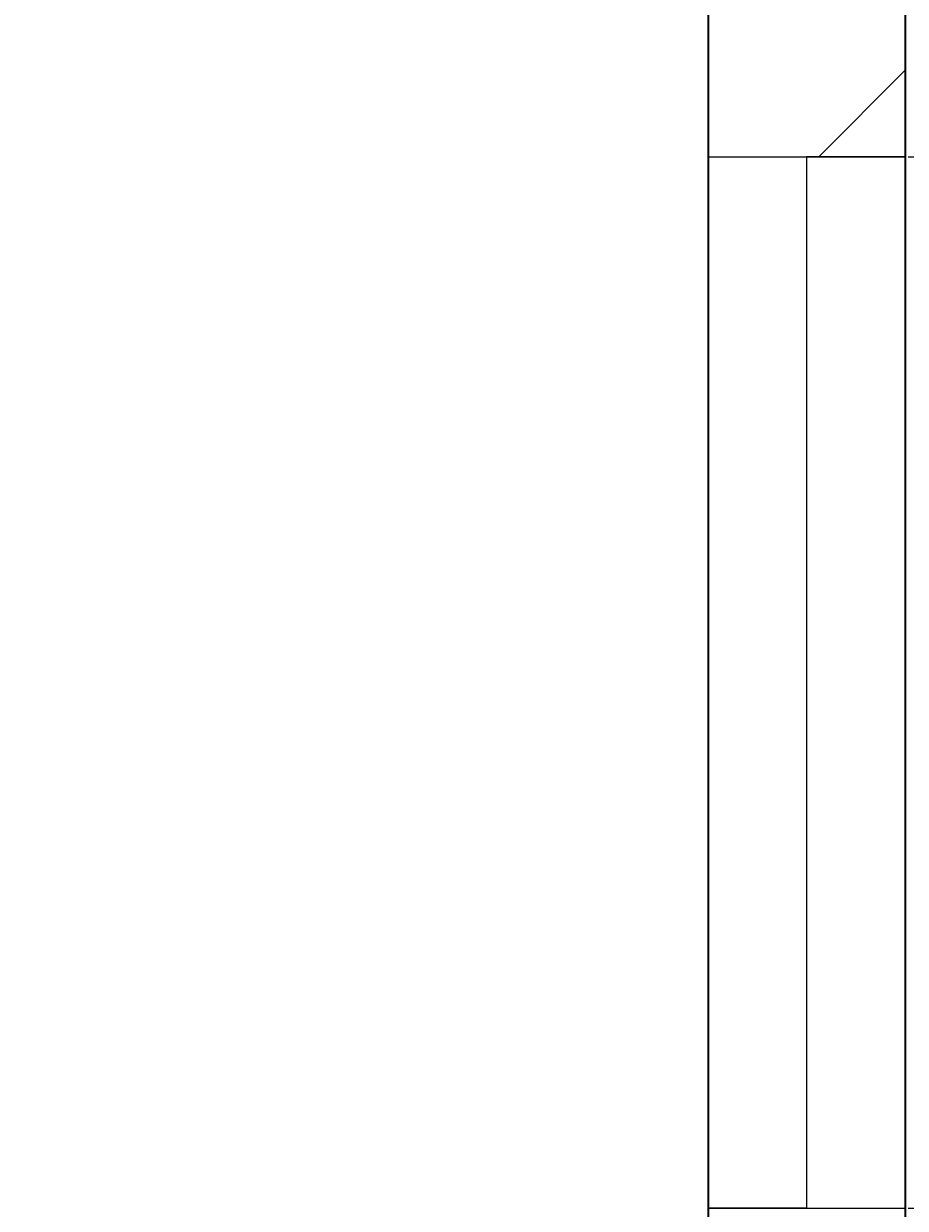
# Model space of a CAD drawing. Units: inches. Extents: x 1962 to 2771, y 1245 to 2660.
# Tile 18 of 114: x 2641 to 2661, y 1665 to 1692. Entities that reach past the tile are written whole.
import ezdxf

# ---------------------------------------------------------------- set-up
doc = ezdxf.new("R2010")
doc.units = ezdxf.units.IN
for name, color, linetype, lineweight in [('A-ANNO-DIMS', 2, 'Continuous', 18), ('A-GLAZ', 4, 'Continuous', 18), ('A-WALL', 7, 'Continuous', 35), ('A-WALL-PATT', 252, 'Continuous', 13)]:
    doc.layers.add(name, color=color, linetype=linetype, lineweight=lineweight)
doc.styles.get("Standard").update_dxf_attribs({"font": 'arial.ttf'})
doc.dimstyles.get("Standard").update_dxf_attribs({"dimtxt": 0.18, "dimasz": 0.18, "dimexe": 0.18, "dimexo": 0.0625, "dimgap": 0.09, "dimtad": 0, "dimtih": 1, "dimtoh": 1, "dimdec": 4, "dimzin": 0, "dimdsep": 46, "dimtxsty": 'Standard', "dimcen": 0.09, "dimadec": 0, "dimazin": 0, "dimtfac": 1, "dimtdec": 4, "dimtofl": 0, "dimtmove": 0, "dimatfit": 3, "dimfxl": 1, "dimtolj": 1, "dimtzin": 0, "dimarcsym": 0})

# ---------------------------------------------------------------- blocks, each defined once
blk = doc.blocks.new('WIN-24IN-A')
for p, q in [((0, 24), (4.5, 24)), ((4.5, 24), (2.25, 24)), ((2.25, 24), (2.25, 0)), ((2.25, 0), (0, 0)), ((0, 0), (4.5, 0))]:
    blk.add_line(p, q)
blk = doc.blocks.new('*D18')
at = {"layer": 'A-ANNO-DIMS', "color": 0, "lineweight": -2, "transparency": 16777216}
for p, q in [((2660.87, 1688.966), (2664.587, 1688.966)), ((2664.407, 1688.786), (2664.407, 1677.147)), ((2664.407, 1665.146), (2664.407, 1676.786)), ((2660.87, 1664.966), (2664.587, 1664.966))]:
    blk.add_line(p, q, dxfattribs=at)
at = {"layer": 'A-ANNO-DIMS', "color": 0, "transparency": 16777216}
for points in [[(2664.377, 1688.786), (2664.437, 1688.786), (2664.407, 1688.966)], [(2664.377, 1665.146), (2664.437, 1665.146), (2664.407, 1664.966)]]:
    blk.add_solid(points, dxfattribs=at)
at = {"layer": 'Defpoints', "color": 0, "transparency": 16777216}
for p in [(2660.807, 1688.966), (2664.407, 1688.966), (2660.807, 1664.966)]:
    blk.add_point(p, dxfattribs=at)
at = {"layer": 'A-ANNO-DIMS', "color": 0, "transparency": 16777216, "insert": (2664.407, 1676.966), "char_height": 0.18, "attachment_point": 5}
blk.add_mtext('\\A1;W1A 24 TYP.', dxfattribs=at)

msp = doc.modelspace()

# ---------------------------------------------------------------- hatches: boundary and pattern name
at = {"layer": 'A-WALL-PATT'}
h = msp.add_hatch(dxfattribs=at)
h.set_pattern_fill('ANSI32', color=256)
h.paths.add_polyline_path([(2090.8074, 2467.3437), (2141.6481, 2467.3437), (2141.6481, 2469.5937), (2141.6481, 2471.8437), (2086.3074, 2471.8437), (2086.3074, 2422.5333), (2090.8074, 2422.5333)])
h.paths.add_polyline_path([(2282.7664, 2471.8437), (2204.8982, 2471.8437), (2204.8982, 2467.3437), (2234.8074, 2467.3437), (2234.8074, 2311.3437), (2228.7492, 2311.3437), (2228.7492, 2306.8437), (2234.8074, 2306.8437), (2331.9227, 2306.8437), (2331.9227, 2309.0937), (2331.9227, 2311.3437), (2239.3074, 2311.3437), (2239.3074, 2467.3437), (2282.7664, 2467.3437), (2282.7664, 2469.5937)])
h.paths.add_polyline_path([(2471.4531, 2519.8437), (2552.011, 2519.8437), (2564.3996, 2519.8437), (2564.3996, 2511.1389), (2568.8996, 2511.1389), (2568.8996, 2524.3437), (2466.9531, 2524.3437), (2466.9531, 2471.8437), (2450.0749, 2471.8437), (2446.4672, 2471.8437), (2446.4672, 2467.3437), (2450.0749, 2467.3437), (2475.9988, 2467.3437), (2475.9988, 2469.5937), (2475.9988, 2471.8437), (2471.4531, 2471.8437)])
h.paths.add_polyline_path([(2575.2231, 2469.5937), (2575.2231, 2471.8437), (2568.8996, 2471.8437), (2568.8996, 2487.1389), (2564.3996, 2487.1389), (2564.3996, 2471.8437), (2556.511, 2471.8437), (2499.2904, 2471.8437), (2499.2904, 2467.3437), (2507.8074, 2467.3437), (2507.8074, 2311.3437), (2414.863, 2311.3437), (2414.863, 2306.8437), (2512.3074, 2306.8437), (2517.0114, 2306.8437), (2517.0114, 2309.0937), (2517.0114, 2311.3437), (2512.3074, 2311.3437), (2512.3074, 2467.3437), (2575.2231, 2467.3437)])
h.paths.add_polyline_path([(2660.8074, 2471.8437), (2600.9602, 2471.8437), (2600.9602, 2467.3437), (2656.3074, 2467.3437), (2656.3074, 2432.5704), (2660.8074, 2432.5704)])
h.paths.add_polyline_path([(2660.8074, 2372.5704), (2656.3074, 2372.5704), (2656.3074, 2311.3437), (2600.276, 2311.3437), (2600.276, 2309.0937), (2600.276, 2306.8437), (2656.3074, 2306.8437), (2656.3074, 2296.2593), (2660.8074, 2296.2593)])
h.paths.add_polyline_path([(2572.3074, 2306.8437), (2577.1385, 2306.8437), (2577.1385, 2311.3437), (2551.082, 2311.3437), (2551.082, 2306.8437), (2567.8074, 2306.8437), (2567.8074, 2258.8437), (2540.0574, 2258.8437), (2540.0574, 2256.5937), (2540.0574, 2254.3437), (2567.8074, 2254.3437), (2656.3074, 2254.3437), (2656.3074, 2236.9085), (2660.8074, 2236.9085), (2660.8074, 2272.2593), (2656.3074, 2272.2593), (2656.3074, 2258.8437), (2572.3074, 2258.8437)])
h.paths.add_polyline_path([(2512.3074, 2254.3437), (2518.8716, 2254.3437), (2518.8716, 2256.5937), (2518.8716, 2258.8437), (2507.8074, 2258.8437), (2507.8074, 2177.8437), (2567.8074, 2177.8437), (2567.8074, 2172.9628), (2572.3074, 2172.9628), (2572.3074, 2177.8437), (2656.3074, 2177.8437), (2656.3074, 2166.4846), (2660.8074, 2166.4846), (2660.8074, 2200.9085), (2656.3074, 2200.9085), (2656.3074, 2182.3437), (2512.3074, 2182.3437)])
h.paths.add_polyline_path([(2656.3074, 2129.8437), (2572.3074, 2129.8437), (2572.3074, 2150.3044), (2570.0574, 2150.3044), (2567.8074, 2150.3044), (2567.8074, 2129.8437), (2507.8074, 2129.8437), (2507.8074, 2116.3027), (2510.0574, 2116.3027), (2512.3074, 2116.3027), (2512.3074, 2125.3437), (2567.8074, 2125.3437), (2572.3074, 2125.3437), (2656.3074, 2125.3437)])
h.paths.add_polyline_path([(2090.8074, 2362.5333), (2086.3074, 2362.5333), (2086.3074, 2298.6242), (2090.8074, 2298.6242), (2090.8074, 2306.8437), (2174.8074, 2306.8437), (2174.8074, 2286.4178), (2179.3074, 2286.4178), (2179.3074, 2306.8437), (2192.8641, 2306.8437), (2192.8641, 2309.0937), (2192.8641, 2311.3437), (2090.8074, 2311.3437)])
h.paths.add_polyline_path([(2209.156, 2258.8437), (2179.3074, 2258.8437), (2179.3074, 2263.2236), (2177.0574, 2263.2236), (2174.8074, 2263.2236), (2174.8074, 2258.8437), (2090.8074, 2258.8437), (2090.8074, 2274.6242), (2086.3074, 2274.6242), (2086.3074, 2238.2967), (2088.5574, 2238.2967), (2090.8074, 2238.2967), (2090.8074, 2254.3437), (2209.156, 2254.3437)])
h.paths.add_polyline_path([(2090.8074, 2177.8437), (2234.8074, 2177.8437), (2234.8074, 2173.1428), (2239.3074, 2173.1428), (2239.3074, 2258.8437), (2230.8442, 2258.8437), (2230.8442, 2256.5937), (2230.8442, 2254.3437), (2234.8074, 2254.3437), (2234.8074, 2182.3437), (2090.8074, 2182.3437), (2090.8074, 2202.2967), (2086.3074, 2202.2967), (2086.3074, 2140.0389), (2090.8074, 2140.0389)])
h.paths.add_polyline_path([(2090.8074, 2080.0389), (2086.3074, 2080.0389), (2086.3074, 2033.8437), (2090.8074, 2033.8437)], flags=17)
h.paths.add_polyline_path([(2244.9405, 2033.8437), (2239.3074, 2033.8437), (2239.3074, 2142.0665), (2237.2592, 2142.0665), (2234.8074, 2142.0665), (2234.8074, 2033.8437), (2090.8074, 2033.8437), (2076.5204, 2033.8437), (2072.0204, 2033.8437), (2072.0204, 2000.4493), (2076.5204, 2000.4493), (2076.5204, 2029.3437), (2090.8074, 2029.3437), (2244.9405, 2029.3437), (2244.9405, 2031.5937)])
h.paths.add_polyline_path([(2234.8074, 1933.3437), (2076.5204, 1933.3437), (2076.5204, 1952.4493), (2074.2704, 1952.4493), (2072.0204, 1952.4493), (2072.0204, 1933.3437), (2072.0204, 1928.8437), (2234.8074, 1928.8437)])
h.paths.add_polyline_path([(2090.8074, 1928.8437), (2086.3074, 1928.8437), (2086.3074, 1906.5013), (2090.8074, 1906.5013)])
h.paths.add_polyline_path([(2090.8074, 1846.5013), (2086.3074, 1846.5013), (2086.3074, 1769.9917), (2088.5574, 1769.9917), (2090.8074, 1769.9917), (2090.8074, 1780.3437), (2234.8074, 1780.3437), (2234.8074, 1708.3437), (2230.3764, 1708.3437), (2230.3764, 1703.8437), (2239.3074, 1703.8437), (2239.3074, 1792.6669), (2237.0574, 1792.6669), (2234.8074, 1792.6669), (2234.8074, 1784.8437), (2090.8074, 1784.8437)])
h.paths.add_polyline_path([(2239.3074, 1928.8437), (2244.9405, 1928.8437), (2244.9405, 1931.0937), (2244.9405, 1933.3437), (2234.8074, 1933.3437), (2234.8074, 1928.8437), (2234.8074, 1825.5949), (2239.3074, 1825.5949)])
h.paths.add_polyline_path([(2148.0425, 1649.0937), (2148.0425, 1651.3437), (2090.8074, 1651.3437), (2090.8074, 1646.8437), (2148.0425, 1646.8437)], flags=0)
h.paths.add_polyline_path([(2207.5601, 1708.3437), (2090.8074, 1708.3437), (2090.8074, 1703.8437), (2174.8074, 1703.8437), (2174.8074, 1651.3437), (2170.4457, 1651.3437), (2170.4457, 1646.8437), (2195.9924, 1646.8437), (2195.9924, 1649.0937), (2195.9924, 1651.3437), (2179.3074, 1651.3437), (2179.3074, 1703.8437), (2207.5601, 1703.8437), (2207.5601, 1706.0937)])
h.paths.add_polyline_path([(2090.8074, 1733.9917), (2086.3074, 1733.9917), (2086.3074, 1696.1032), (2088.5574, 1696.1032), (2090.8074, 1696.1032)])
h.paths.add_polyline_path([(2090.8074, 1672.1032), (2086.3074, 1672.1032), (2086.3074, 1600.3335), (2090.8074, 1600.3335)])
h.paths.add_polyline_path([(2090.8074, 1540.3335), (2086.3074, 1540.3335), (2086.3074, 1486.3437), (2139.6766, 1486.3437), (2139.6766, 1490.8437), (2090.8074, 1490.8437)])
h.paths.add_polyline_path([(2302.3876, 1490.8437), (2239.3074, 1490.8437), (2239.3074, 1646.8437), (2335.9994, 1646.8437), (2335.9994, 1651.3437), (2229.884, 1651.3437), (2229.884, 1646.8437), (2234.8074, 1646.8437), (2234.8074, 1490.8437), (2202.7103, 1490.8437), (2202.7103, 1488.5937), (2202.7103, 1486.3437), (2275.0699, 1486.3437), (2275.0699, 1475.772), (2279.5699, 1475.772), (2279.5699, 1486.3437), (2302.3876, 1486.3437)])
h.paths.add_polyline_path([(2279.5699, 1451.772), (2275.0699, 1451.772), (2275.0699, 1438.3437), (2174.8074, 1438.3437), (2174.8074, 1486.3437), (2179.7922, 1486.3437), (2179.7922, 1490.8437), (2163.3585, 1490.8437), (2163.3585, 1488.5937), (2163.3585, 1486.3437), (2170.3074, 1486.3437), (2170.3074, 1433.8437), (2279.5699, 1433.8437)])
h.paths.add_polyline_path([(2427.2363, 1490.8437), (2375.8074, 1490.8437), (2375.8074, 1646.8437), (2381.6401, 1646.8437), (2381.6401, 1651.3437), (2365.887, 1651.3437), (2365.887, 1649.0937), (2365.887, 1646.8437), (2371.3074, 1646.8437), (2371.3074, 1490.8437), (2327.5627, 1490.8437), (2327.5627, 1488.5937), (2327.5627, 1486.3437), (2371.3074, 1486.3437), (2371.3074, 1433.8437), (2375.8074, 1433.8437), (2375.8074, 1486.3437), (2427.2363, 1486.3437)])
h.paths.add_polyline_path([(2512.3074, 1646.8437), (2519.4351, 1646.8437), (2519.4351, 1649.0937), (2519.4351, 1651.3437), (2507.8074, 1651.3437), (2416.0063, 1651.3437), (2416.0063, 1649.0937), (2416.0063, 1646.8437), (2507.8074, 1646.8437), (2507.8074, 1490.8437), (2497.0532, 1490.8437), (2497.0532, 1488.5937), (2497.0532, 1486.3437), (2574.9344, 1486.3437), (2574.9344, 1476.0181), (2579.4344, 1476.0181), (2579.4344, 1486.3437), (2584.4872, 1486.3437), (2584.3074, 1490.8437), (2512.3074, 1490.8437)])
h.paths.add_polyline_path([(2470.5091, 1486.3437), (2473.9767, 1486.3437), (2473.9767, 1490.8437), (2449.6605, 1490.8437), (2449.6605, 1488.5937), (2449.6605, 1486.3437), (2466.0091, 1486.3437), (2466.0091, 1433.8437), (2470.5091, 1433.8437), (2579.4344, 1433.8437), (2579.4344, 1452.0181), (2574.9344, 1452.0181), (2574.9344, 1438.3437), (2554.5091, 1438.3437), (2470.5091, 1438.3437)])
h.paths.add_polyline_path([(2656.3074, 1490.8437), (2611.86, 1490.8437), (2611.86, 1486.3437), (2656.3074, 1486.3437)])
h.paths.add_polyline_path([(2660.8074, 1532.7007), (2658.5574, 1532.7007), (2656.3074, 1532.7007), (2656.3074, 1486.3437), (2660.8074, 1486.3437)])
h.paths.add_polyline_path([(2660.8074, 1664.9663), (2656.3074, 1664.9663), (2656.3074, 1651.3437), (2602.2313, 1651.3437), (2602.2313, 1646.8437), (2656.3074, 1646.8437), (2656.3074, 1592.7007), (2660.8074, 1592.7007)])
h.paths.add_polyline_path([(2660.8074, 1724.5221), (2656.3074, 1724.5221), (2656.3074, 1703.8437), (2542.4725, 1703.8437), (2542.4725, 1699.3437), (2567.8074, 1699.3437), (2567.8074, 1651.3437), (2552.7766, 1651.3437), (2552.7766, 1649.0937), (2552.7766, 1646.8437), (2577.2878, 1646.8437), (2577.2878, 1649.0937), (2577.2878, 1651.3437), (2572.3074, 1651.3437), (2572.3074, 1699.3437), (2656.3074, 1699.3437), (2656.3074, 1688.9663), (2660.8074, 1688.9663)])
h.paths.add_polyline_path([(2660.8074, 1880.6524), (2656.3074, 1880.6524), (2656.3074, 1832.8437), (2512.3074, 1832.8437), (2512.3074, 1837.8959), (2507.8074, 1837.8959), (2507.8074, 1828.3437), (2567.8074, 1828.3437), (2567.8074, 1804.3437), (2572.3074, 1804.3437), (2572.3074, 1828.3437), (2656.3074, 1828.3437), (2656.3074, 1818.6778), (2660.8074, 1818.6778)])
h.paths.add_polyline_path([(2660.8074, 1794.6778), (2656.3074, 1794.6778), (2656.3074, 1780.3437), (2572.3074, 1780.3437), (2572.3074, 1783.0303), (2570.0574, 1783.0303), (2567.8074, 1783.0303), (2567.8074, 1780.3437), (2507.8074, 1780.3437), (2507.8074, 1699.3437), (2517.8858, 1699.3437), (2517.8858, 1701.5937), (2517.8858, 1703.8437), (2512.3074, 1703.8437), (2512.3074, 1775.8437), (2656.3074, 1775.8437), (2656.3074, 1760.5221), (2660.8074, 1760.5221)])
h.paths.add_polyline_path([(2660.8074, 1981.3437), (2660.8074, 2020.2808), (2658.5574, 2020.2808), (2656.3074, 2020.2808), (2656.3074, 1981.3437), (2512.3074, 1981.3437), (2512.3074, 2086.6996), (2507.8074, 2086.6996), (2507.8074, 1981.3437), (2375.8074, 1981.3437), (2375.8074, 1986.8505), (2373.5574, 1986.8505), (2371.3074, 1986.8505), (2371.3074, 1973.2607), (2375.8074, 1973.2607), (2375.8074, 1976.8437), (2507.8074, 1976.8437), (2507.8074, 1865.4281), (2510.0574, 1865.4281), (2512.3074, 1865.4281), (2512.3074, 1976.8437), (2660.8074, 1976.8437)])
h.paths.add_polyline_path([(2375.8074, 1940.297), (2373.5574, 1940.297), (2371.3074, 1940.297), (2371.3074, 1933.3437), (2278.4434, 1933.3437), (2278.4434, 1928.8437), (2371.3074, 1928.8437), (2371.3074, 1651.3437), (2375.8074, 1651.3437)])
h.paths.add_polyline_path([(2660.8074, 1976.8437), (2656.3074, 1976.8437), (2656.3074, 1940.6524), (2660.8074, 1940.6524)], flags=17)
h.paths.add_polyline_path([(2660.8074, 2142.4846), (2656.3074, 2142.4846), (2656.3074, 2080.2808), (2660.8074, 2080.2808)])
h.paths.add_polyline_path([(2381.4189, 2311.3437), (2375.8074, 2311.3437), (2375.8074, 2467.3437), (2424.7242, 2467.3437), (2424.7242, 2469.5937), (2424.7242, 2471.8437), (2375.8074, 2471.8437), (2375.8074, 2524.3437), (2371.3074, 2524.3437), (2371.3074, 2471.8437), (2307.2097, 2471.8437), (2307.2097, 2467.3437), (2371.3074, 2467.3437), (2371.3074, 2311.3437), (2366.8901, 2311.3437), (2366.8901, 2306.8437), (2371.3074, 2306.8437), (2371.3074, 2033.8437), (2279.6589, 2033.8437), (2279.6589, 2029.3437), (2371.3074, 2029.3437), (2371.3074, 2014.2598), (2375.8074, 2014.2598), (2375.8074, 2306.8437), (2381.4189, 2306.8437)])
h.paths.add_polyline_path([(2263.3074, 2524.3437), (2170.3074, 2524.3437), (2170.3074, 2519.8437), (2170.3074, 2471.8437), (2165.0312, 2471.8437), (2165.0312, 2467.3437), (2179.6721, 2467.3437), (2179.6721, 2469.5161), (2179.6721, 2471.8437), (2174.8074, 2471.8437), (2174.8074, 2519.8437), (2258.8074, 2519.8437), (2258.8074, 2511.6436), (2263.3074, 2511.6436)])
h.paths.add_polyline_path([(2245.0232, 1361.4123), (2492.9468, 1361.4123), (2492.9468, 1398.505), (2245.0232, 1398.505)], flags=9)
h.paths.add_polyline_path([(2388.1434, 2086.6936), (2425.0704, 2086.6936), (2425.0704, 2105.3509), (2388.1434, 2105.3509)], flags=9)
h.paths.add_polyline_path([(2404.922, 2242.6744), (2445.7337, 2242.6744), (2445.7337, 2261.3318), (2404.922, 2261.3318)], flags=9)
h.paths.add_polyline_path([(2269.4107, 2156.7935), (2306.3378, 2156.7935), (2306.3378, 2175.4508), (2269.4107, 2175.4508)], flags=9)
h.paths.add_polyline_path([(2269.3277, 2233.4343), (2306.2547, 2233.4343), (2306.2547, 2252.0917), (2269.3277, 2252.0917)], flags=9)
h.paths.add_polyline_path([(2431.6052, 2320.6922), (2470.4456, 2320.6922), (2470.4456, 2339.3495), (2431.6052, 2339.3495)], flags=25)
h.paths.add_polyline_path([(2249.6902, 2315.7608), (2288.5306, 2315.7608), (2288.5306, 2334.4182), (2249.6902, 2334.4182)], flags=25)
h.paths.add_polyline_path([(2096.9301, 2314.3181), (2135.7704, 2314.3181), (2135.7704, 2332.9755), (2096.9301, 2332.9755)], flags=25)
h.paths.add_polyline_path([(2134.3475, 2285.7089), (2161.4655, 2285.7089), (2161.4655, 2304.3662), (2134.3475, 2304.3662)], flags=9)
h.paths.add_polyline_path([(2126.5155, 2209.4076), (2159.9227, 2209.4076), (2159.9227, 2228.065), (2126.5155, 2228.065)], flags=25)
h.paths.add_polyline_path([(2110.5753, 2141.5299), (2149.4157, 2141.5299), (2149.4157, 2160.1872), (2110.5753, 2160.1872)], flags=25)
h.paths.add_polyline_path([(2249.8618, 1968.3317), (2286.3966, 1968.3317), (2286.3966, 1986.989), (2249.8618, 1986.989)], flags=9)
h.paths.add_polyline_path([(2395.9507, 1777.0051), (2436.7624, 1777.0051), (2436.7624, 1795.6625), (2395.9507, 1795.6625)], flags=9)
h.paths.add_polyline_path([(2398.5259, 1888.5651), (2435.0062, 1888.5651), (2435.0062, 1907.2224), (2398.5259, 1907.2224)], flags=25)
h.paths.add_polyline_path([(2259.3506, 1728.3559), (2296.2776, 1728.3559), (2296.2776, 1747.0132), (2259.3506, 1747.0132)], flags=9)
h.paths.add_polyline_path([(2271.3698, 1845.268), (2308.2968, 1845.268), (2308.2968, 1863.9253), (2271.3698, 1863.9253)], flags=9)
h.paths.add_polyline_path([(2120.9355, 1786.3027), (2159.7759, 1786.3027), (2159.7759, 1804.9601), (2120.9355, 1804.9601)], flags=25)
h.paths.add_polyline_path([(2121.3164, 1732.1043), (2154.7236, 1732.1043), (2154.7236, 1750.7616), (2121.3164, 1750.7616)], flags=25)
h.paths.add_polyline_path([(2118.3706, 1678.8997), (2147.5282, 1678.8997), (2147.5282, 1697.557), (2118.3706, 1697.557)], flags=25)
h.paths.add_polyline_path([(2385.9227, 1493.557), (2424.763, 1493.557), (2424.763, 1512.2143), (2385.9227, 1512.2143)], flags=25)
h.paths.add_polyline_path([(2248.7058, 1500.0256), (2287.5462, 1500.0256), (2287.5462, 1518.6829), (2248.7058, 1518.6829)], flags=25)
h.paths.add_polyline_path([(2104.1669, 1617.3771), (2143.0073, 1617.3771), (2143.0073, 1636.0344), (2104.1669, 1636.0344)], flags=9)
h.paths.add_polyline_path([(2096.0714, 1447.8824), (2137.3845, 1447.8824), (2137.3845, 1458.1859), (2096.0714, 1458.1859)], flags=9)
h.paths.add_polyline_path([(2180.6114, 1440.325), (2209.7689, 1440.325), (2209.7689, 1458.9823), (2180.6114, 1458.9823)], flags=25)
h.paths.add_polyline_path([(2316.1698, 1447.9637), (2357.4829, 1447.9637), (2357.4829, 1458.2673), (2316.1698, 1458.2673)], flags=9)
h.paths.add_polyline_path([(2397.6187, 1447.9637), (2438.9318, 1447.9637), (2438.9318, 1458.2673), (2397.6187, 1458.2673)], flags=9)
h.paths.add_polyline_path([(2473.0778, 1439.5953), (2502.2354, 1439.5953), (2502.2354, 1458.2527), (2473.0778, 1458.2527)], flags=25)
h.paths.add_polyline_path([(2589.7027, 1447.8819), (2631.0158, 1447.8819), (2631.0158, 1458.1855), (2589.7027, 1458.1855)], flags=9)
h.paths.add_polyline_path([(2522.4009, 1497.5285), (2561.2413, 1497.5285), (2561.2413, 1516.1859), (2522.4009, 1516.1859)], flags=25)
h.paths.add_polyline_path([(2579.6565, 1671.3482), (2608.8141, 1671.3482), (2608.8141, 1690.0056), (2579.6565, 1690.0056)], flags=25)
h.paths.add_polyline_path([(2544.7038, 1725.5064), (2578.1111, 1725.5064), (2578.1111, 1744.1637), (2544.7038, 1744.1637)], flags=25)
h.paths.add_polyline_path([(2578.1191, 1807.472), (2607.2766, 1807.472), (2607.2766, 1826.1293), (2578.1191, 1826.1293)], flags=25)
h.paths.add_polyline_path([(2595.0614, 1835.1839), (2633.9018, 1835.1839), (2633.9018, 1853.8413), (2595.0614, 1853.8413)], flags=25)
h.paths.add_polyline_path([(2567.0097, 2097.7035), (2605.8501, 2097.7035), (2605.8501, 2116.3609), (2567.0097, 2116.3609)], flags=9)
h.paths.add_polyline_path([(2586.644, 2134.6454), (2615.8015, 2134.6454), (2615.8015, 2153.3027), (2586.644, 2153.3027)], flags=9)
h.paths.add_polyline_path([(2544.6185, 2212.6783), (2578.0258, 2212.6783), (2578.0258, 2231.3356), (2544.6185, 2231.3356)], flags=25)
h.paths.add_polyline_path([(2577.0273, 2256.9023), (2606.1849, 2256.9023), (2606.1849, 2275.5597), (2577.0273, 2275.5597)], flags=24)
h.paths.add_polyline_path([(2605.2683, 2315.2821), (2644.1087, 2315.2821), (2644.1087, 2333.9395), (2605.2683, 2333.9395)], flags=25)
h.paths.add_polyline_path([(2583.1244, 2496.1815), (2624.4375, 2496.1815), (2624.4375, 2506.4851), (2583.1244, 2506.4851)], flags=9)
h.paths.add_polyline_path([(2474.761, 2497.0823), (2503.9185, 2497.0823), (2503.9185, 2515.7397), (2474.761, 2515.7397)], flags=25)
h.paths.add_polyline_path([(2387.5787, 2494.2563), (2428.902, 2494.2563), (2428.902, 2504.5598), (2387.5787, 2504.5598)], flags=9)
h.paths.add_polyline_path([(2300.1657, 2500.1564), (2341.4788, 2500.1564), (2341.4788, 2510.46), (2300.1657, 2510.46)], flags=25)
h.paths.add_polyline_path([(2176.8589, 2497.5843), (2206.0165, 2497.5843), (2206.0165, 2516.2416), (2176.8589, 2516.2416)], flags=25)
h.paths.add_polyline_path([(2097.4668, 2494.9762), (2138.7799, 2494.9762), (2138.7799, 2505.2798), (2097.4668, 2505.2798)], flags=9)

# ---------------------------------------------------------------- linework, layer by layer
at = {"layer": 'A-WALL'}
for p, q in [((2660.8074, 1976.8437), (2660.8074, 1486.3437)), ((2656.3074, 1699.3437), (2656.3074, 1651.3437))]:
    msp.add_line(p, q, dxfattribs=at)

# ---------------------------------------------------------------- block references
at = {"layer": 'A-GLAZ'}
msp.add_blockref('WIN-24IN-A', (2656.3074, 1664.9663), dxfattribs=at)

# ---------------------------------------------------------------- dimensions: what is measured, and where the dimension line sits
at = {"layer": 'A-ANNO-DIMS'}
dim = msp.add_linear_dim(base=(2664.4074, 1688.9663), p1=(2660.8074, 1664.9663), p2=(2660.8074, 1688.9663), angle=90, text='W1A <> TYP.', dimstyle='Standard', override={"dimdec": 0, "dimlfac": 1, "dimrnd": 0, "dimzin": 0, "dimdsep": 46, "dimlunit": 2}, dxfattribs=at)
dim.commit()
dim.dimension.update_dxf_attribs({"geometry": '*D18', "text_midpoint": (2664.4074, 1676.9663)})

doc.saveas('drawing.dxf')
